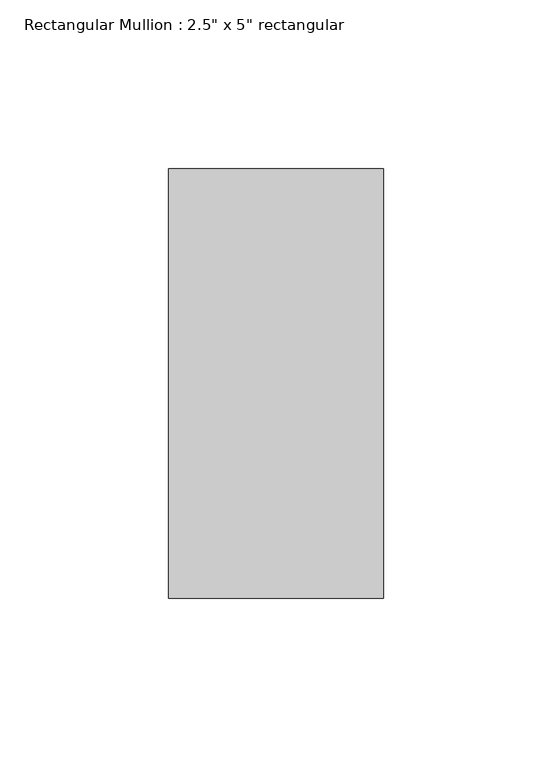
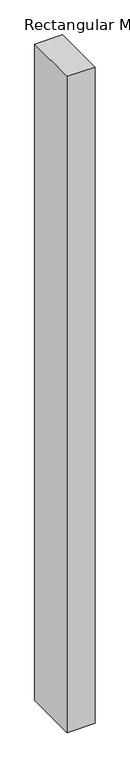
"""IFC4 building model written with IfcOpenShell, lengths in millimetres: member geometry."""

from ifc_helpers import new_model, si_unit, frame, origin, place, context, project, spatial, polyline, outline, extrude, source, transform, mapped, element, save


def member_db0015e1(model_context):
    return source(origin(), model_context, "Body", "SweptSolid", [
        extrude(outline(polyline([(0.0, 63.5), (0.0, -63.5), (-63.5, -63.5), (-63.5, 63.5), (0.0, 63.5)])), frame((0.0, 0.0, -1574.2288132), z_axis=(0.0, 0.0, 1.0), x_axis=(1.0, 0.0, 0.0)), (0.0, 0.0, 1.0), 1574.2288132),
    ])


if __name__ == "__main__":
    model = new_model("IFC4")
    model_context = context("Model", 3, world=origin())
    ifc_project = project(units=[si_unit("LENGTHUNIT", "METRE", prefix="MILLI")], contexts=[model_context])
    site = spatial("IfcSite", under=ifc_project)
    building = spatial("IfcBuilding", under=site)
    placement = place(None, origin())
    member_shape = member_db0015e1(model_context)
    element("IfcMember", 1, ObjectType="Rectangular Mullion : 2.5\" x 5\" rectangular", at=placement, inside=building, context=model_context, shape_type="MappedRepresentation", body=[
        mapped(member_shape, transform((0.0, 0.0, 0.0), x_axis=(1.0, 0.0, 0.0), y_axis=(0.0, 1.0, 0.0), z_axis=(0.0, 0.0, 1.0))),
    ])
    save(model, "model.ifc")

# Revit data of these elements
# Type "Rectangular Mullion : 2.5\" x 5\" rectangular"
#   built-in parameter 1007304 = 0.416667 (stored number, unit not read)
#   built-in parameter 1007301 = 0.104167 (stored number, unit not read)
#   built-in parameter 1007300 = 0.104167 (stored number, unit not read)
# Element 1 (IfcMember, "Rectangular Mullion : 2.5\" x 5\" rectangular")
#   Materials on its faces: "Aluminum"
# Materials
#   "Aluminum": class "Metal", colour RGB 247 247 247, transparency 0, Description = "Aluminum 6061", Cost = 0
